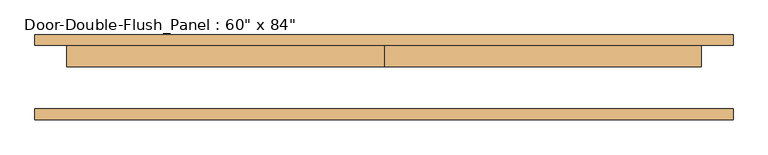
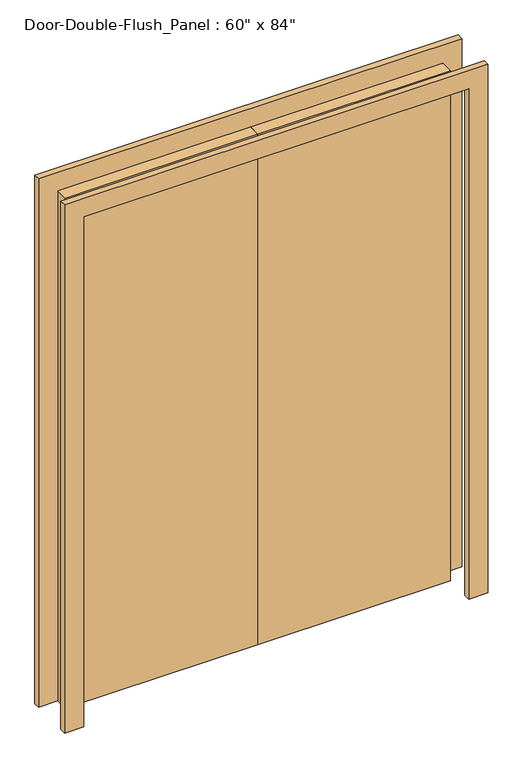
"""IFC4 building model written with IfcOpenShell, lengths in millimetres: door geometry."""

from ifc_helpers import new_model, si_unit, frame, origin, origin_with_axes, place, context, project, spatial, polyline, outline, extrude, source, transform, mapped, element, save


def door_a09c2f77(model_context):
    return source(origin(), model_context, "Body", "SweptSolid", [
        extrude(outline(polyline([(2133.6, -762.0), (2133.6, 762.0), (0.0, 762.0), (0.0, 838.2), (2209.8, 838.2), (2209.8, -838.2), (0.0, -838.2), (0.0, -762.0), (2133.6, -762.0)])), frame((0.0, 76.2, 0.0), z_axis=(0.0, 1.0, 0.0), x_axis=(0.0, 0.0, 1.0)), (0.0, 0.0, 1.0), 25.4),
        extrude(outline(polyline([(2133.6, -762.0), (2133.6, 762.0), (0.0, 762.0), (0.0, 838.2), (2209.8, 838.2), (2209.8, -838.2), (0.0, -838.2), (0.0, -762.0), (2133.6, -762.0)])), frame((0.0, -101.6, 0.0), z_axis=(0.0, 1.0, 0.0), x_axis=(0.0, 0.0, 1.0)), (0.0, 0.0, 1.0), 25.4),
        extrude(outline(polyline([(-762.0, 76.2), (0.0, 76.2), (0.0, 25.4), (-762.0, 25.4), (-762.0, 76.2)])), origin_with_axes(), (0.0, 0.0, 1.0), 2133.6),
        extrude(outline(polyline([(0.0, 76.2), (762.0, 76.2), (762.0, 25.4), (0.0, 25.4), (0.0, 76.2)])), origin_with_axes(), (0.0, 0.0, 1.0), 2133.6),
    ])


if __name__ == "__main__":
    model = new_model("IFC4")
    model_context = context("Model", 3, world=origin())
    ifc_project = project(units=[si_unit("LENGTHUNIT", "METRE", prefix="MILLI")], contexts=[model_context])
    site = spatial("IfcSite", under=ifc_project)
    building = spatial("IfcBuilding", under=site)
    placement = place(None, origin())
    door_shape = door_a09c2f77(model_context)
    element("IfcDoor", 1, ObjectType="Door-Double-Flush_Panel : 60\" x 84\"", at=placement, inside=building, context=model_context, shape_type="MappedRepresentation", body=[
        mapped(door_shape, transform((0.0, 0.0, 0.0), x_axis=(1.0, 0.0, 0.0), y_axis=(0.0, 1.0, 0.0), z_axis=(0.0, 0.0, 1.0))),
    ])
    save(model, "model.ifc")

# Revit data of these elements
# Type "Door-Double-Flush_Panel : 60\" x 84\""
#   Type Mark = "9"
#   Construction Type Id = "DOOR"
#   Assembly Code = "C1020"
#   Analytic Construction = "Wooden"
#   Thickness = 0' - 2"
#   Thermal Resistance (R) = 2.5876 (h·ft²·°F)/BTU
#   Swing Angle [instance default] = 90.00°
#   Panel Width = 2' - 6"
#   Heat Transfer Coefficient (U) = 0.3865 BTU/(h·ft²·°F)
#   Height = 7' - 0"
#   Trim Projection Ext = 0' - 1"
#   Trim Projection Int = 0' - 1"
#   Trim Width = 0' - 3"
#   Width = 5' - 0"
#   Define Thermal Properties by = 1
#   Panel Material = Wood - Birch - Solid Stained Light Low Gloss
#   Trim Material = Paint - Sienna
#   Visual Light Transmittance = 0
#   Solar Heat Gain Coefficient = 0
#   Function = (empty or 0)
#   Wall Closure = (empty or 0)
# Element 1 (IfcDoor, "Door-Double-Flush_Panel : 60\" x 84\"")
#   Materials on its faces: "Paint - Sienna", "Wood - Birch - Solid Stained Light Low Gloss"
# Materials
#   "Wood - Birch - Solid Stained Light Low Gloss": class "Wood", colour RGB 210 159 95, transparency 0, Cost = 0
#   "Paint - Sienna": colour RGB 118 70 51, transparency 0, Cost = 0
